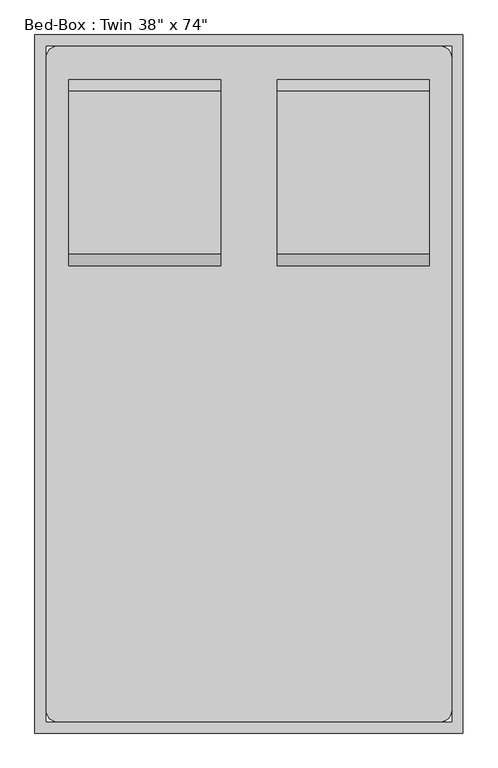
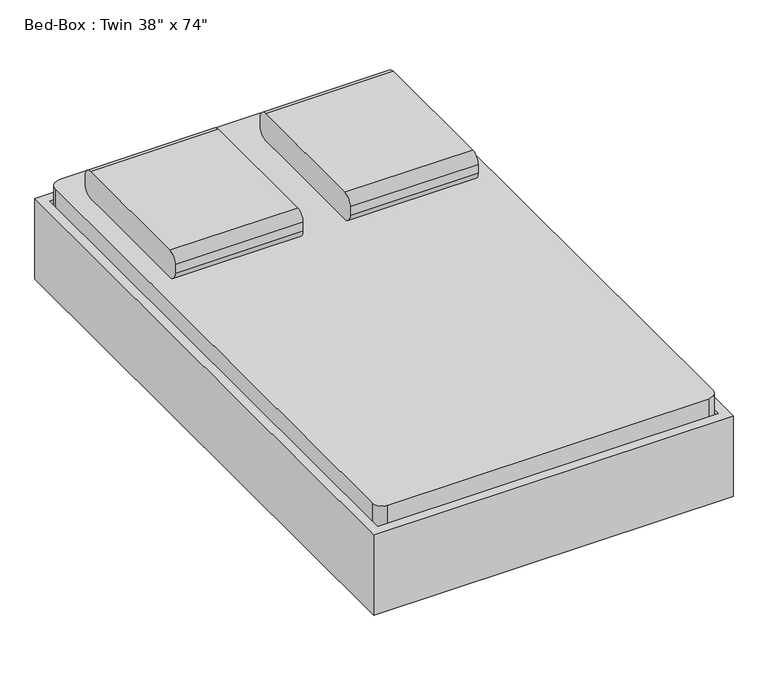
"""IFC4 building model written with IfcOpenShell, lengths in millimetres: furniture geometry."""

from ifc_helpers import new_model, si_unit, point, frame, frame_2d, origin, place, context, project, spatial, polyline, circle_curve, trimmed, segment, composite_curve, outline, extrude, source, transform, mapped, element, save
from ifc_brep_helpers import plane_surface, cylinder_surface, revolved_surface, advanced_brep


def furniture_631c00ae(model_context):
    return source(origin(), model_context, "Body", "SolidModel", [
        extrude(outline(composite_curve([segment(polyline([(425.9704918, 406.4), (57.6704918, 406.4)]), True, "CONTINUOUS"), segment(trimmed(circle_curve(frame_2d((57.6704918, 431.8)), 25.4), [point((57.6704918, 406.4))], [point((32.2704918, 431.8))], False, "CARTESIAN"), True, "CONTINUOUS"), segment(polyline([(32.2704918, 431.8), (32.2704918, 457.2)]), True, "CONTINUOUS"), segment(trimmed(circle_curve(frame_2d((57.6704918, 457.2)), 25.4), [point((32.2704918, 457.2))], [point((57.6704918, 482.6))], False, "CARTESIAN"), True, "CONTINUOUS"), segment(polyline([(57.6704918, 482.6), (425.9704918, 482.6)]), True, "CONTINUOUS"), segment(trimmed(circle_curve(frame_2d((425.9704918, 457.2)), 25.4), [point((425.9704918, 482.6))], [point((451.3704918, 457.2))], False, "CARTESIAN"), True, "CONTINUOUS"), segment(polyline([(451.3704918, 457.2), (451.3704918, 431.8)]), True, "CONTINUOUS"), segment(trimmed(circle_curve(frame_2d((425.9704918, 431.8)), 25.4), [point((451.3704918, 431.8))], [point((425.9704918, 406.4))], False, "CARTESIAN"), True, "CONTINUOUS")], self_intersect=False)), frame((402.652459, 0.0, 0.0), z_axis=(1.0, 0.0, 0.0), x_axis=(0.0, 1.0, 0.0)), (0.0, 0.0, 1.0), 342.9),
        extrude(outline(composite_curve([segment(polyline([(425.9704918, 406.4), (57.6704918, 406.4)]), True, "CONTINUOUS"), segment(trimmed(circle_curve(frame_2d((57.6704918, 431.8)), 25.4), [point((57.6704918, 406.4))], [point((32.2704918, 431.8))], False, "CARTESIAN"), True, "CONTINUOUS"), segment(polyline([(32.2704918, 431.8), (32.2704918, 457.2)]), True, "CONTINUOUS"), segment(trimmed(circle_curve(frame_2d((57.6704918, 457.2)), 25.4), [point((32.2704918, 457.2))], [point((57.6704918, 482.6))], False, "CARTESIAN"), True, "CONTINUOUS"), segment(polyline([(57.6704918, 482.6), (425.9704918, 482.6)]), True, "CONTINUOUS"), segment(trimmed(circle_curve(frame_2d((425.9704918, 457.2)), 25.4), [point((425.9704918, 482.6))], [point((451.3704918, 457.2))], False, "CARTESIAN"), True, "CONTINUOUS"), segment(polyline([(451.3704918, 457.2), (451.3704918, 431.8)]), True, "CONTINUOUS"), segment(trimmed(circle_curve(frame_2d((425.9704918, 431.8)), 25.4), [point((451.3704918, 431.8))], [point((425.9704918, 406.4))], False, "CARTESIAN"), True, "CONTINUOUS")], self_intersect=False)), frame((-67.247541, 0.0, 0.0), z_axis=(1.0, 0.0, 0.0), x_axis=(0.0, 1.0, 0.0)), (0.0, 0.0, 1.0), 342.9),
        advanced_brep(
        [(-117.7231784, 298.9704918, 177.8), (-117.7231784, 222.7704918, 177.8), (-117.7231784, 222.7704918, 196.85), (-117.7231784, 298.9704918, 196.85), (-66.9231784, 298.9704918, 177.8), (-66.9231784, 222.7704918, 177.8), (-54.7869899, 222.7704918, 196.85), (-54.7869899, 298.9704918, 196.85), (9.1476901, 298.9704918, 14.6654962), (9.1476901, 222.7704918, 14.6654962), (26.4128534, 222.7704918, 22.716374), (26.4128534, 298.9704918, 22.716374), (32.1679079, 222.7704918, 0.0), (32.1679079, 298.9704918, 0.0), (32.1679079, 222.7704918, 19.05), (32.1679079, 298.9704918, 19.05), (110.7804138, 298.9704918, 0.0), (110.7804138, 222.7704918, 0.0), (110.7804138, 222.7704918, 19.05), (110.7804138, 298.9704918, 19.05), (123.4804138, 222.7704918, 3.4029547), (123.4804138, 298.9704918, 3.4029547), (113.9554138, 222.7704918, 19.9007387), (113.9554138, 298.9704918, 19.9007387), (183.577459, 298.9704918, 38.1), (183.577459, 222.7704918, 38.1), (178.4730269, 222.7704918, 57.15), (178.4730269, 298.9704918, 57.15), (495.0518216, 298.9704918, 38.1), (495.0518216, 222.7704918, 38.1), (500.1562537, 222.7704918, 57.15), (500.1562537, 298.9704918, 57.15), (555.1488669, 298.9704918, 3.4029547), (555.1488669, 222.7704918, 3.4029547), (564.6738669, 222.7704918, 19.9007387), (564.6738669, 298.9704918, 19.9007387), (567.8488669, 222.7704918, 0.0), (567.8488669, 298.9704918, 0.0), (567.8488669, 222.7704918, 19.05), (567.8488669, 298.9704918, 19.05), (646.4613728, 298.9704918, 0.0), (646.4613728, 222.7704918, 0.0), (646.4613728, 222.7704918, 19.05), (646.4613728, 298.9704918, 19.05), (669.4815906, 222.7704918, 14.6654962), (669.4815906, 298.9704918, 14.6654962), (652.2164272, 222.7704918, 22.716374), (652.2164272, 298.9704918, 22.716374), (745.552459, 298.9704918, 177.8), (745.552459, 222.7704918, 177.8), (733.4162705, 222.7704918, 196.85), (733.4162705, 298.9704918, 196.85), (796.352459, 298.9704918, 177.8), (796.352459, 298.9704918, 196.85), (796.352459, 222.7704918, 196.85), (796.352459, 222.7704918, 177.8)],
        [
            (0, 1),
            (1, 2),
            (2, 3),
            (3, 0),
            (0, 4),
            (4, 5),
            (5, 1),
            (5, 6),
            (6, 2),
            (6, 7),
            (7, 3),
            (7, 4),
            (4, 8),
            (8, 9),
            (9, 5),
            (9, 10),
            (10, 6),
            (10, 11),
            (11, 7),
            (11, 8),
            (12, 9, circle_curve(frame((32.1679079, 222.7704918, 25.4), z_axis=(0.0, 1.0, 0.0), x_axis=(-0.9063077870366486, 0.0, -0.42261826174070233)), 25.4)),
            (8, 13, circle_curve(frame((32.1679079, 298.9704918, 25.4), z_axis=(0.0, -1.0, 0.0), x_axis=(-0.9063077870366486, 0.0, -0.42261826174070233)), 25.4)),
            (13, 12),
            (14, 10, circle_curve(frame((32.1679079, 222.7704918, 25.4), z_axis=(0.0, 1.0, 0.0), x_axis=(-0.9063077870366486, 0.0, -0.42261826174070233)), 6.35)),
            (12, 14),
            (15, 11, circle_curve(frame((32.1679079, 298.9704918, 25.4), z_axis=(0.0, 1.0, 0.0), x_axis=(-0.9063077870366486, 0.0, -0.42261826174070233)), 6.35)),
            (14, 15),
            (15, 13),
            (13, 16),
            (16, 17),
            (17, 12),
            (17, 18),
            (18, 14),
            (18, 19),
            (19, 15),
            (19, 16),
            (20, 17, circle_curve(frame((110.7804138, 222.7704918, 25.4), z_axis=(0.0, 1.0, 0.0), x_axis=(0.0, 0.0, -1.0)), 25.4)),
            (16, 21, circle_curve(frame((110.7804138, 298.9704918, 25.4), z_axis=(0.0, -1.0, 0.0), x_axis=(0.0, 0.0, -1.0)), 25.4)),
            (21, 20),
            (22, 18, circle_curve(frame((110.7804138, 222.7704918, 25.4), z_axis=(0.0, 1.0, 0.0), x_axis=(0.0, 0.0, -1.0)), 6.35)),
            (20, 22),
            (23, 19, circle_curve(frame((110.7804138, 298.9704918, 25.4), z_axis=(0.0, 1.0, 0.0), x_axis=(0.0, 0.0, -1.0)), 6.35)),
            (22, 23),
            (23, 21),
            (21, 24),
            (24, 25),
            (25, 20),
            (25, 26),
            (26, 22),
            (26, 27),
            (27, 23),
            (27, 24),
            (24, 28),
            (28, 29),
            (29, 25),
            (29, 30),
            (30, 26),
            (30, 31),
            (31, 27),
            (31, 28),
            (28, 32),
            (32, 33),
            (33, 29),
            (33, 34),
            (34, 30),
            (34, 35),
            (35, 31),
            (35, 32),
            (36, 33, circle_curve(frame((567.8488669, 222.7704918, 25.4), z_axis=(0.0, 1.0, 0.0), x_axis=(-0.5000000000000463, 0.0, -0.8660254037844118)), 25.4)),
            (32, 37, circle_curve(frame((567.8488669, 298.9704918, 25.4), z_axis=(0.0, -1.0, 0.0), x_axis=(-0.5000000000000463, 0.0, -0.8660254037844118)), 25.4)),
            (37, 36),
            (38, 34, circle_curve(frame((567.8488669, 222.7704918, 25.4), z_axis=(0.0, 1.0, 0.0), x_axis=(-0.5000000000000463, 0.0, -0.8660254037844118)), 6.35)),
            (36, 38),
            (39, 35, circle_curve(frame((567.8488669, 298.9704918, 25.4), z_axis=(0.0, 1.0, 0.0), x_axis=(-0.5000000000000463, 0.0, -0.8660254037844118)), 6.35)),
            (38, 39),
            (39, 37),
            (37, 40),
            (40, 41),
            (41, 36),
            (41, 42),
            (42, 38),
            (42, 43),
            (43, 39),
            (43, 40),
            (44, 41, circle_curve(frame((646.4613728, 222.7704918, 25.4), z_axis=(0.0, 1.0, 0.0), x_axis=(0.0, 0.0, -1.0)), 25.4)),
            (40, 45, circle_curve(frame((646.4613728, 298.9704918, 25.4), z_axis=(0.0, -1.0, 0.0), x_axis=(0.0, 0.0, -1.0)), 25.4)),
            (45, 44),
            (46, 42, circle_curve(frame((646.4613728, 222.7704918, 25.4), z_axis=(0.0, 1.0, 0.0), x_axis=(0.0, 0.0, -1.0)), 6.35)),
            (44, 46),
            (47, 43, circle_curve(frame((646.4613728, 298.9704918, 25.4), z_axis=(0.0, 1.0, 0.0), x_axis=(0.0, 0.0, -1.0)), 6.35)),
            (46, 47),
            (47, 45),
            (45, 48),
            (48, 49),
            (49, 44),
            (49, 50),
            (50, 46),
            (50, 51),
            (51, 47),
            (51, 48),
            (52, 53),
            (53, 54),
            (54, 55),
            (55, 52),
            (48, 52),
            (55, 49),
            (54, 50),
            (53, 51),
        ],
        [
            plane_surface(frame((-117.7231784, 552.9704918, -152.9490627), z_axis=(-1.0, 0.0, 0.0), x_axis=(0.0, 1.0, 0.0))),
            plane_surface(frame((-117.7231784, 298.9704918, 177.8), z_axis=(0.0, 0.0, -1.0), x_axis=(1.0, 0.0, 0.0))),
            plane_surface(frame((-117.7231784, 222.7704918, 177.8), z_axis=(0.0, -1.0, 0.0), x_axis=(1.0, 0.0, 0.0))),
            plane_surface(frame((-117.7231784, 222.7704918, 196.85), z_axis=(0.0, 0.0, 1.0), x_axis=(1.0, 0.0, 0.0))),
            plane_surface(frame((-117.7231784, 298.9704918, 196.85), z_axis=(0.0, 1.0, 0.0), x_axis=(1.0, 0.0, 0.0))),
            plane_surface(frame((-66.9231784, 298.9704918, 177.8), z_axis=(-0.9063077870366486, 0.0, -0.42261826174070244), x_axis=(0.42261826174070244, 0.0, -0.9063077870366486))),
            plane_surface(frame((-66.9231784, 222.7704918, 177.8), z_axis=(0.0, -1.0000000000000002, 0.0), x_axis=(0.4226182617407026, 0.0, -0.9063077870366486))),
            plane_surface(frame((-54.7869899, 222.7704918, 196.85), z_axis=(0.9063077870366485, 0.0, 0.4226182617407026), x_axis=(0.4226182617407026, 0.0, -0.9063077870366485))),
            plane_surface(frame((-54.7869899, 298.9704918, 196.85), z_axis=(0.0, 1.0000000000000002, 0.0), x_axis=(0.4226182617407026, 0.0, -0.9063077870366486))),
            cylinder_surface(frame((32.1679079, 552.9704918, 25.4), z_axis=(0.0, -1.0, 0.0), x_axis=(-0.9063077870366486, 0.0, -0.42261826174070233)), 25.4),
            plane_surface(frame((32.1679079, 222.7704918, 25.4), z_axis=(0.0, -1.0, 0.0), x_axis=(-0.9063077870366486, 0.0, -0.42261826174070233))),
            revolved_surface(polyline([(26.412853452317286, 222.7704918, 22.71637403794654), (26.412853452317286, 298.9704918, 22.71637403794654)]), (32.1679079, 552.9704918, 25.4), (0.0, -1.0, 0.0)),
            plane_surface(frame((32.1679079, 298.9704918, 25.4), z_axis=(0.0, 1.0, 0.0), x_axis=(-0.9063077870366486, 0.0, -0.42261826174070233))),
            plane_surface(frame((32.1679079, 298.9704918, 0.0), z_axis=(0.0, 0.0, -1.0), x_axis=(1.0, 0.0, 0.0))),
            plane_surface(frame((32.1679079, 222.7704918, 0.0), z_axis=(0.0, -1.0, 0.0), x_axis=(1.0, 0.0, 0.0))),
            plane_surface(frame((32.1679079, 222.7704918, 19.05), z_axis=(0.0, 0.0, 1.0), x_axis=(1.0, 0.0, 0.0))),
            plane_surface(frame((32.1679079, 298.9704918, 19.05), z_axis=(0.0, 1.0, 0.0), x_axis=(1.0, 0.0, 0.0))),
            cylinder_surface(frame((110.7804138, 552.9704918, 25.4), z_axis=(0.0, -1.0, 0.0), x_axis=(0.0, 0.0, -1.0)), 25.4),
            plane_surface(frame((110.7804138, 222.7704918, 25.4), z_axis=(0.0, -1.0, 0.0), x_axis=(0.0, 0.0, -1.0))),
            revolved_surface(polyline([(110.7804138, 222.7704918, 19.049999999999997), (110.7804138, 298.9704918, 19.049999999999997)]), (110.7804138, 552.9704918, 25.4), (0.0, -1.0, 0.0)),
            plane_surface(frame((110.7804138, 298.9704918, 25.4), z_axis=(0.0, 1.0, 0.0), x_axis=(0.0, 0.0, -1.0))),
            plane_surface(frame((123.4804138, 298.9704918, 3.4029547), z_axis=(0.49999999999987804, 0.0, -0.8660254037845091), x_axis=(0.8660254037845091, 0.0, 0.49999999999987804))),
            plane_surface(frame((123.4804138, 222.7704918, 3.4029547), z_axis=(0.0, -1.0, 0.0), x_axis=(0.8660254037845093, 0.0, 0.49999999999987765))),
            plane_surface(frame((113.9554138, 222.7704918, 19.9007387), z_axis=(-0.49999999999987815, 0.0, 0.8660254037845091), x_axis=(0.8660254037845091, 0.0, 0.49999999999987815))),
            plane_surface(frame((113.9554138, 298.9704918, 19.9007387), z_axis=(0.0, 1.0, 0.0), x_axis=(0.8660254037845092, 0.0, 0.49999999999987776))),
            plane_surface(frame((183.577459, 298.9704918, 38.1), z_axis=(0.0, 0.0, -1.0), x_axis=(1.0, 0.0, 0.0))),
            plane_surface(frame((183.577459, 222.7704918, 38.1), z_axis=(0.0, -1.0, 0.0), x_axis=(1.0, 0.0, 0.0))),
            plane_surface(frame((178.4730269, 222.7704918, 57.15), z_axis=(0.0, 0.0, 1.0), x_axis=(1.0, 0.0, 0.0))),
            plane_surface(frame((178.4730269, 298.9704918, 57.15), z_axis=(0.0, 1.0, 0.0), x_axis=(1.0, 0.0, 0.0))),
            plane_surface(frame((495.0518216, 298.9704918, 38.1), z_axis=(-0.5000000000000461, 0.0, -0.8660254037844122), x_axis=(0.8660254037844122, 0.0, -0.5000000000000461))),
            plane_surface(frame((495.0518216, 222.7704918, 38.1), z_axis=(0.0, -1.0, 0.0), x_axis=(0.8660254037844125, 0.0, -0.5000000000000454))),
            plane_surface(frame((500.1562537, 222.7704918, 57.15), z_axis=(0.5000000000000456, 0.0, 0.8660254037844124), x_axis=(0.8660254037844124, 0.0, -0.5000000000000456))),
            plane_surface(frame((500.1562537, 298.9704918, 57.15), z_axis=(0.0, 1.0, 0.0), x_axis=(0.8660254037844127, 0.0, -0.5000000000000449))),
            cylinder_surface(frame((567.8488669, 552.9704918, 25.4), z_axis=(0.0, -1.0, 0.0), x_axis=(-0.5000000000000463, 0.0, -0.8660254037844118)), 25.4),
            plane_surface(frame((567.8488669, 222.7704918, 25.4), z_axis=(0.0, -1.0000000000000002, 0.0), x_axis=(-0.5000000000000464, 0.0, -0.866025403784412))),
            revolved_surface(polyline([(564.6738668999997, 222.7704918, 19.90073868596898), (564.6738668999997, 298.9704918, 19.90073868596898)]), (567.8488669, 552.9704918, 25.4), (0.0, -1.0, 0.0)),
            plane_surface(frame((567.8488669, 298.9704918, 25.4), z_axis=(0.0, 1.0000000000000002, 0.0), x_axis=(-0.5000000000000464, 0.0, -0.866025403784412))),
            plane_surface(frame((567.8488669, 298.9704918, 0.0), z_axis=(0.0, 0.0, -1.0), x_axis=(1.0, 0.0, 0.0))),
            plane_surface(frame((567.8488669, 222.7704918, 0.0), z_axis=(0.0, -1.0, 0.0), x_axis=(1.0, 0.0, 0.0))),
            plane_surface(frame((567.8488669, 222.7704918, 19.05), z_axis=(0.0, 0.0, 1.0), x_axis=(1.0, 0.0, 0.0))),
            plane_surface(frame((567.8488669, 298.9704918, 19.05), z_axis=(0.0, 1.0, 0.0), x_axis=(1.0, 0.0, 0.0))),
            cylinder_surface(frame((646.4613728, 552.9704918, 25.4), z_axis=(0.0, -1.0, 0.0), x_axis=(0.0, 0.0, -1.0)), 25.4),
            plane_surface(frame((646.4613728, 222.7704918, 25.4), z_axis=(0.0, -1.0, 0.0), x_axis=(0.0, 0.0, -1.0))),
            revolved_surface(polyline([(646.4613728, 222.7704918, 19.049999999999997), (646.4613728, 298.9704918, 19.049999999999997)]), (646.4613728, 552.9704918, 25.4), (0.0, -1.0, 0.0)),
            plane_surface(frame((646.4613728, 298.9704918, 25.4), z_axis=(0.0, 1.0, 0.0), x_axis=(0.0, 0.0, -1.0))),
            plane_surface(frame((669.4815906, 298.9704918, 14.6654962), z_axis=(0.90630778703668, 0.0, -0.42261826174063516), x_axis=(0.42261826174063516, 0.0, 0.90630778703668))),
            plane_surface(frame((669.4815906, 222.7704918, 14.6654962), z_axis=(0.0, -1.0, 0.0), x_axis=(0.422618261740635, 0.0, 0.90630778703668))),
            plane_surface(frame((652.2164272, 222.7704918, 22.716374), z_axis=(-0.9063077870366799, 0.0, 0.42261826174063544), x_axis=(0.42261826174063544, 0.0, 0.9063077870366799))),
            plane_surface(frame((652.2164272, 298.9704918, 22.716374), z_axis=(0.0, 1.0, 0.0), x_axis=(0.4226182617406361, 0.0, 0.9063077870366795))),
            plane_surface(frame((796.352459, 552.9704918, -152.9490627), z_axis=(1.0, 0.0, 0.0), x_axis=(0.0, 1.0, 0.0))),
            plane_surface(frame((745.552459, 298.9704918, 177.8), z_axis=(0.0, 0.0, -1.0), x_axis=(1.0, 0.0, 0.0))),
            plane_surface(frame((745.552459, 222.7704918, 177.8), z_axis=(0.0, -1.0, 0.0), x_axis=(1.0, 0.0, 0.0))),
            plane_surface(frame((733.4162705, 222.7704918, 196.85), z_axis=(0.0, 0.0, 1.0), x_axis=(1.0, 0.0, 0.0))),
            plane_surface(frame((733.4162705, 298.9704918, 196.85), z_axis=(0.0, 1.0, 0.0), x_axis=(1.0, 0.0, 0.0))),
        ],
        [
            (0, [[1, 2, 3, 4]]),
            (1, [[-1, 5, 6, 7]]),
            (2, [[-2, -7, 8, 9]]),
            (3, [[-3, -9, 10, 11]]),
            (4, [[-4, -11, 12, -5]]),
            (5, [[-6, 13, 14, 15]]),
            (6, [[-8, -15, 16, 17]]),
            (7, [[-10, -17, 18, 19]]),
            (8, [[-12, -19, 20, -13]]),
            (9, [[21, -14, 22, 23]]),
            (10, [[24, -16, -21, 25]]),
            (11, [[26, -18, -24, 27]]),
            (12, [[-22, -20, -26, 28]]),
            (13, [[-23, 29, 30, 31]]),
            (14, [[-25, -31, 32, 33]]),
            (15, [[-27, -33, 34, 35]]),
            (16, [[-28, -35, 36, -29]]),
            (17, [[37, -30, 38, 39]]),
            (18, [[40, -32, -37, 41]]),
            (19, [[42, -34, -40, 43]]),
            (20, [[-38, -36, -42, 44]]),
            (21, [[-39, 45, 46, 47]]),
            (22, [[-41, -47, 48, 49]]),
            (23, [[-43, -49, 50, 51]]),
            (24, [[-44, -51, 52, -45]]),
            (25, [[-46, 53, 54, 55]]),
            (26, [[-48, -55, 56, 57]]),
            (27, [[-50, -57, 58, 59]]),
            (28, [[-52, -59, 60, -53]]),
            (29, [[-54, 61, 62, 63]]),
            (30, [[-56, -63, 64, 65]]),
            (31, [[-58, -65, 66, 67]]),
            (32, [[-60, -67, 68, -61]]),
            (33, [[69, -62, 70, 71]]),
            (34, [[72, -64, -69, 73]]),
            (35, [[74, -66, -72, 75]]),
            (36, [[-70, -68, -74, 76]]),
            (37, [[-71, 77, 78, 79]]),
            (38, [[-73, -79, 80, 81]]),
            (39, [[-75, -81, 82, 83]]),
            (40, [[-76, -83, 84, -77]]),
            (41, [[85, -78, 86, 87]]),
            (42, [[88, -80, -85, 89]]),
            (43, [[90, -82, -88, 91]]),
            (44, [[-86, -84, -90, 92]]),
            (45, [[-87, 93, 94, 95]]),
            (46, [[-89, -95, 96, 97]]),
            (47, [[-91, -97, 98, 99]]),
            (48, [[-92, -99, 100, -93]]),
            (49, [[101, 102, 103, 104]]),
            (50, [[-94, 105, -104, 106]]),
            (51, [[-96, -106, -103, 107]]),
            (52, [[-98, -107, -102, 108]]),
            (53, [[-100, -108, -101, -105]]),
        ],
    ),
        extrude(outline(composite_curve([segment(polyline([(-92.647541, 527.5704918), (770.952459, 527.5704918)]), True, "CONTINUOUS"), segment(trimmed(circle_curve(frame_2d((770.952459, 502.1704918)), 25.4), [point((770.952459, 527.5704918))], [point((796.352459, 502.1704918))], False, "CARTESIAN"), True, "CONTINUOUS"), segment(polyline([(796.352459, 502.1704918), (796.352459, -971.0295082)]), True, "CONTINUOUS"), segment(trimmed(circle_curve(frame_2d((770.952459, -971.0295082)), 25.4), [point((796.352459, -971.0295082))], [point((770.952459, -996.4295082))], False, "CARTESIAN"), True, "CONTINUOUS"), segment(polyline([(770.952459, -996.4295082), (-92.647541, -996.4295082)]), True, "CONTINUOUS"), segment(trimmed(circle_curve(frame_2d((-92.647541, -971.0295082)), 25.4), [point((-92.647541, -996.4295082))], [point((-118.047541, -971.0295082))], False, "CARTESIAN"), True, "CONTINUOUS"), segment(polyline([(-118.047541, -971.0295082), (-118.047541, 502.1704918)]), True, "CONTINUOUS"), segment(trimmed(circle_curve(frame_2d((-92.647541, 502.1704918)), 25.4), [point((-118.047541, 502.1704918))], [point((-92.647541, 527.5704918))], False, "CARTESIAN"), True, "CONTINUOUS")], self_intersect=False)), frame((0.0, 0.0, 203.2), z_axis=(0.0, 0.0, 1.0), x_axis=(1.0, 0.0, 0.0)), (0.0, 0.0, 1.0), 203.2),
        advanced_brep(
        [(-118.047541, -717.0295082, 196.85), (-118.047541, -717.0295082, 177.8), (-118.047541, -793.2295082, 177.8), (-118.047541, -793.2295082, 196.85), (-55.1113525, -717.0295082, 196.85), (-67.247541, -717.0295082, 177.8), (-67.247541, -793.2295082, 177.8), (-55.1113525, -793.2295082, 196.85), (26.0884908, -717.0295082, 22.716374), (8.8233275, -717.0295082, 14.6654962), (8.8233275, -793.2295082, 14.6654962), (26.0884908, -793.2295082, 22.716374), (31.8435453, -717.0295082, 0.0), (31.8435453, -717.0295082, 19.05), (31.8435453, -793.2295082, 0.0), (31.8435453, -793.2295082, 19.05), (110.4560511, -717.0295082, 19.05), (110.4560511, -717.0295082, 0.0), (110.4560511, -793.2295082, 0.0), (110.4560511, -793.2295082, 19.05), (123.1560511, -717.0295082, 3.4029547), (113.6310511, -717.0295082, 19.9007387), (123.1560511, -793.2295082, 3.4029547), (113.6310511, -793.2295082, 19.9007387), (178.1486643, -717.0295082, 57.15), (183.2530964, -717.0295082, 38.1), (183.2530964, -793.2295082, 38.1), (178.1486643, -793.2295082, 57.15), (500.1562537, -717.0295082, 57.15), (495.0518216, -717.0295082, 38.1), (495.0518216, -793.2295082, 38.1), (500.1562537, -793.2295082, 57.15), (564.6738669, -717.0295082, 19.9007387), (555.1488669, -717.0295082, 3.4029547), (555.1488669, -793.2295082, 3.4029547), (564.6738669, -793.2295082, 19.9007387), (567.8488669, -717.0295082, 0.0), (567.8488669, -717.0295082, 19.05), (567.8488669, -793.2295082, 0.0), (567.8488669, -793.2295082, 19.05), (646.4613728, -717.0295082, 19.05), (646.4613728, -717.0295082, 0.0), (646.4613728, -793.2295082, 0.0), (646.4613728, -793.2295082, 19.05), (669.4815906, -717.0295082, 14.6654962), (652.2164272, -717.0295082, 22.716374), (669.4815906, -793.2295082, 14.6654962), (652.2164272, -793.2295082, 22.716374), (733.4162705, -717.0295082, 196.85), (745.552459, -717.0295082, 177.8), (745.552459, -793.2295082, 177.8), (733.4162705, -793.2295082, 196.85), (796.352459, -717.0295082, 196.85), (796.352459, -793.2295082, 196.85), (796.352459, -793.2295082, 177.8), (796.352459, -717.0295082, 177.8)],
        [
            (0, 1),
            (1, 2),
            (2, 3),
            (3, 0),
            (0, 4),
            (4, 5),
            (5, 1),
            (5, 6),
            (6, 2),
            (6, 7),
            (7, 3),
            (7, 4),
            (4, 8),
            (8, 9),
            (9, 5),
            (9, 10),
            (10, 6),
            (10, 11),
            (11, 7),
            (11, 8),
            (12, 9, circle_curve(frame((31.8435453, -717.0295082, 25.4), z_axis=(0.0, 1.0, 0.0), x_axis=(-0.906307787036663, 0.0, -0.4226182617406713)), 25.4)),
            (8, 13, circle_curve(frame((31.8435453, -717.0295082, 25.4), z_axis=(0.0, -1.0, 0.0), x_axis=(-0.906307787036663, 0.0, -0.4226182617406713)), 6.35)),
            (13, 12),
            (14, 10, circle_curve(frame((31.8435453, -793.2295082, 25.4), z_axis=(0.0, 1.0, 0.0), x_axis=(-0.906307787036663, 0.0, -0.4226182617406713)), 25.4)),
            (12, 14),
            (15, 11, circle_curve(frame((31.8435453, -793.2295082, 25.4), z_axis=(0.0, 1.0, 0.0), x_axis=(-0.906307787036663, 0.0, -0.4226182617406713)), 6.35)),
            (14, 15),
            (15, 13),
            (13, 16),
            (16, 17),
            (17, 12),
            (17, 18),
            (18, 14),
            (18, 19),
            (19, 15),
            (19, 16),
            (20, 17, circle_curve(frame((110.4560511, -717.0295082, 25.4), z_axis=(0.0, 1.0, 0.0), x_axis=(0.0, 0.0, -1.0)), 25.4)),
            (16, 21, circle_curve(frame((110.4560511, -717.0295082, 25.4), z_axis=(0.0, -1.0, 0.0), x_axis=(0.0, 0.0, -1.0)), 6.35)),
            (21, 20),
            (22, 18, circle_curve(frame((110.4560511, -793.2295082, 25.4), z_axis=(0.0, 1.0, 0.0), x_axis=(0.0, 0.0, -1.0)), 25.4)),
            (20, 22),
            (23, 19, circle_curve(frame((110.4560511, -793.2295082, 25.4), z_axis=(0.0, 1.0, 0.0), x_axis=(0.0, 0.0, -1.0)), 6.35)),
            (22, 23),
            (23, 21),
            (21, 24),
            (24, 25),
            (25, 20),
            (25, 26),
            (26, 22),
            (26, 27),
            (27, 23),
            (27, 24),
            (24, 28),
            (28, 29),
            (29, 25),
            (29, 30),
            (30, 26),
            (30, 31),
            (31, 27),
            (31, 28),
            (28, 32),
            (32, 33),
            (33, 29),
            (33, 34),
            (34, 30),
            (34, 35),
            (35, 31),
            (35, 32),
            (36, 33, circle_curve(frame((567.8488669, -717.0295082, 25.4), z_axis=(0.0, 1.0, 0.0), x_axis=(-0.5000000000000479, 0.0, -0.866025403784411)), 25.4)),
            (32, 37, circle_curve(frame((567.8488669, -717.0295082, 25.4), z_axis=(0.0, -1.0, 0.0), x_axis=(-0.5000000000000479, 0.0, -0.866025403784411)), 6.35)),
            (37, 36),
            (38, 34, circle_curve(frame((567.8488669, -793.2295082, 25.4), z_axis=(0.0, 1.0, 0.0), x_axis=(-0.5000000000000479, 0.0, -0.866025403784411)), 25.4)),
            (36, 38),
            (39, 35, circle_curve(frame((567.8488669, -793.2295082, 25.4), z_axis=(0.0, 1.0, 0.0), x_axis=(-0.5000000000000479, 0.0, -0.866025403784411)), 6.35)),
            (38, 39),
            (39, 37),
            (37, 40),
            (40, 41),
            (41, 36),
            (41, 42),
            (42, 38),
            (42, 43),
            (43, 39),
            (43, 40),
            (44, 41, circle_curve(frame((646.4613728, -717.0295082, 25.4), z_axis=(0.0, 1.0, 0.0), x_axis=(0.0, 0.0, -1.0)), 25.4)),
            (40, 45, circle_curve(frame((646.4613728, -717.0295082, 25.4), z_axis=(0.0, -1.0, 0.0), x_axis=(0.0, 0.0, -1.0)), 6.35)),
            (45, 44),
            (46, 42, circle_curve(frame((646.4613728, -793.2295082, 25.4), z_axis=(0.0, 1.0, 0.0), x_axis=(0.0, 0.0, -1.0)), 25.4)),
            (44, 46),
            (47, 43, circle_curve(frame((646.4613728, -793.2295082, 25.4), z_axis=(0.0, 1.0, 0.0), x_axis=(0.0, 0.0, -1.0)), 6.35)),
            (46, 47),
            (47, 45),
            (45, 48),
            (48, 49),
            (49, 44),
            (49, 50),
            (50, 46),
            (50, 51),
            (51, 47),
            (51, 48),
            (52, 53),
            (53, 54),
            (54, 55),
            (55, 52),
            (48, 52),
            (55, 49),
            (54, 50),
            (53, 51),
        ],
        [
            plane_surface(frame((-118.047541, -1021.8295082, -127.5947323), z_axis=(-1.0, 0.0, 0.0), x_axis=(0.0, 1.0, 0.0))),
            plane_surface(frame((-118.047541, -717.0295082, 196.85), z_axis=(0.0, 1.0, 0.0), x_axis=(1.0, 0.0, 0.0))),
            plane_surface(frame((-118.047541, -717.0295082, 177.8), z_axis=(0.0, 0.0, -1.0), x_axis=(1.0, 0.0, 0.0))),
            plane_surface(frame((-118.047541, -793.2295082, 177.8), z_axis=(0.0, -1.0, 0.0), x_axis=(1.0, 0.0, 0.0))),
            plane_surface(frame((-118.047541, -793.2295082, 196.85), z_axis=(0.0, 0.0, 1.0), x_axis=(1.0, 0.0, 0.0))),
            plane_surface(frame((-55.1113525, -717.0295082, 196.85), z_axis=(0.0, 1.0000000000000002, 0.0), x_axis=(0.42261826174067113, 0.0, -0.9063077870366633))),
            plane_surface(frame((-67.247541, -717.0295082, 177.8), z_axis=(-0.9063077870366633, 0.0, -0.42261826174067096), x_axis=(0.42261826174067096, 0.0, -0.9063077870366633))),
            plane_surface(frame((-67.247541, -793.2295082, 177.8), z_axis=(0.0, -1.0, 0.0), x_axis=(0.4226182617406711, 0.0, -0.9063077870366631))),
            plane_surface(frame((-55.1113525, -793.2295082, 196.85), z_axis=(0.906307787036663, 0.0, 0.4226182617406714), x_axis=(0.4226182617406714, 0.0, -0.906307787036663))),
            plane_surface(frame((31.8435453, -717.0295082, 25.4), z_axis=(0.0, 1.0, 0.0), x_axis=(-0.906307787036663, 0.0, -0.4226182617406713))),
            cylinder_surface(frame((31.8435453, -1021.8295082, 25.4), z_axis=(0.0, -1.0, 0.0), x_axis=(-0.906307787036663, 0.0, -0.4226182617406713)), 25.4),
            plane_surface(frame((31.8435453, -793.2295082, 25.4), z_axis=(0.0, -1.0, 0.0), x_axis=(-0.906307787036663, 0.0, -0.4226182617406713))),
            revolved_surface(polyline([(26.08849085231719, -793.2295082, 22.716374037946736), (26.08849085231719, -717.0295082, 22.716374037946736)]), (31.8435453, -1021.8295082, 25.4), (0.0, -1.0, 0.0)),
            plane_surface(frame((31.8435453, -717.0295082, 19.05), z_axis=(0.0, 1.0, 0.0), x_axis=(1.0, 0.0, 0.0))),
            plane_surface(frame((31.8435453, -717.0295082, 0.0), z_axis=(0.0, 0.0, -1.0), x_axis=(1.0, 0.0, 0.0))),
            plane_surface(frame((31.8435453, -793.2295082, 0.0), z_axis=(0.0, -1.0, 0.0), x_axis=(1.0, 0.0, 0.0))),
            plane_surface(frame((31.8435453, -793.2295082, 19.05), z_axis=(0.0, 0.0, 1.0), x_axis=(1.0, 0.0, 0.0))),
            plane_surface(frame((110.4560511, -717.0295082, 25.4), z_axis=(0.0, 1.0, 0.0), x_axis=(0.0, 0.0, -1.0))),
            cylinder_surface(frame((110.4560511, -1021.8295082, 25.4), z_axis=(0.0, -1.0, 0.0), x_axis=(0.0, 0.0, -1.0)), 25.4),
            plane_surface(frame((110.4560511, -793.2295082, 25.4), z_axis=(0.0, -1.0, 0.0), x_axis=(0.0, 0.0, -1.0))),
            revolved_surface(polyline([(110.4560511, -793.2295082, 19.049999999999997), (110.4560511, -717.0295082, 19.049999999999997)]), (110.4560511, -1021.8295082, 25.4), (0.0, -1.0, 0.0)),
            plane_surface(frame((113.6310511, -717.0295082, 19.9007387), z_axis=(0.0, 1.0, 0.0), x_axis=(0.8660254037844787, 0.0, 0.4999999999999308))),
            plane_surface(frame((123.1560511, -717.0295082, 3.4029547), z_axis=(0.4999999999999308, 0.0, -0.8660254037844786), x_axis=(0.8660254037844786, 0.0, 0.4999999999999308))),
            plane_surface(frame((123.1560511, -793.2295082, 3.4029547), z_axis=(0.0, -1.0, 0.0), x_axis=(0.8660254037844786, 0.0, 0.49999999999993083))),
            plane_surface(frame((113.6310511, -793.2295082, 19.9007387), z_axis=(-0.4999999999999306, 0.0, 0.8660254037844788), x_axis=(0.8660254037844788, 0.0, 0.4999999999999306))),
            plane_surface(frame((178.1486643, -717.0295082, 57.15), z_axis=(0.0, 1.0, 0.0), x_axis=(1.0, 0.0, 0.0))),
            plane_surface(frame((183.2530964, -717.0295082, 38.1), z_axis=(0.0, 0.0, -1.0), x_axis=(1.0, 0.0, 0.0))),
            plane_surface(frame((183.2530964, -793.2295082, 38.1), z_axis=(0.0, -1.0, 0.0), x_axis=(1.0, 0.0, 0.0))),
            plane_surface(frame((178.1486643, -793.2295082, 57.15), z_axis=(0.0, 0.0, 1.0), x_axis=(1.0, 0.0, 0.0))),
            plane_surface(frame((500.1562537, -717.0295082, 57.15), z_axis=(0.0, 1.0, 0.0), x_axis=(0.8660254037844095, 0.0, -0.5000000000000506))),
            plane_surface(frame((495.0518216, -717.0295082, 38.1), z_axis=(-0.5000000000000508, 0.0, -0.8660254037844094), x_axis=(0.8660254037844094, 0.0, -0.5000000000000508))),
            plane_surface(frame((495.0518216, -793.2295082, 38.1), z_axis=(0.0, -1.0, 0.0), x_axis=(0.8660254037844094, 0.0, -0.5000000000000506))),
            plane_surface(frame((500.1562537, -793.2295082, 57.15), z_axis=(0.5000000000000505, 0.0, 0.8660254037844095), x_axis=(0.8660254037844095, 0.0, -0.5000000000000505))),
            plane_surface(frame((567.8488669, -717.0295082, 25.4), z_axis=(0.0, 1.0000000000000002, 0.0), x_axis=(-0.500000000000048, 0.0, -0.8660254037844111))),
            cylinder_surface(frame((567.8488669, -1021.8295082, 25.4), z_axis=(0.0, -1.0, 0.0), x_axis=(-0.5000000000000479, 0.0, -0.866025403784411)), 25.4),
            plane_surface(frame((567.8488669, -793.2295082, 25.4), z_axis=(0.0, -1.0000000000000002, 0.0), x_axis=(-0.500000000000048, 0.0, -0.8660254037844111))),
            revolved_surface(polyline([(564.6738668999997, -793.2295082, 19.90073868596899), (564.6738668999997, -717.0295082, 19.90073868596899)]), (567.8488669, -1021.8295082, 25.4), (0.0, -1.0, 0.0)),
            plane_surface(frame((567.8488669, -717.0295082, 19.05), z_axis=(0.0, 1.0, 0.0), x_axis=(1.0, 0.0, 0.0))),
            plane_surface(frame((567.8488669, -717.0295082, 0.0), z_axis=(0.0, 0.0, -1.0), x_axis=(1.0, 0.0, 0.0))),
            plane_surface(frame((567.8488669, -793.2295082, 0.0), z_axis=(0.0, -1.0, 0.0), x_axis=(1.0, 0.0, 0.0))),
            plane_surface(frame((567.8488669, -793.2295082, 19.05), z_axis=(0.0, 0.0, 1.0), x_axis=(1.0, 0.0, 0.0))),
            plane_surface(frame((646.4613728, -717.0295082, 25.4), z_axis=(0.0, 1.0, 0.0), x_axis=(0.0, 0.0, -1.0))),
            cylinder_surface(frame((646.4613728, -1021.8295082, 25.4), z_axis=(0.0, -1.0, 0.0), x_axis=(0.0, 0.0, -1.0)), 25.4),
            plane_surface(frame((646.4613728, -793.2295082, 25.4), z_axis=(0.0, -1.0, 0.0), x_axis=(0.0, 0.0, -1.0))),
            revolved_surface(polyline([(646.4613728, -793.2295082, 19.049999999999997), (646.4613728, -717.0295082, 19.049999999999997)]), (646.4613728, -1021.8295082, 25.4), (0.0, -1.0, 0.0)),
            plane_surface(frame((652.2164272, -717.0295082, 22.716374), z_axis=(0.0, 1.0000000000000002, 0.0), x_axis=(0.42261826174054085, 0.0, 0.906307787036724))),
            plane_surface(frame((669.4815906, -717.0295082, 14.6654962), z_axis=(0.9063077870367241, 0.0, -0.4226182617405405), x_axis=(0.4226182617405405, 0.0, 0.9063077870367241))),
            plane_surface(frame((669.4815906, -793.2295082, 14.6654962), z_axis=(0.0, -1.0, 0.0), x_axis=(0.42261826174054046, 0.0, 0.9063077870367241))),
            plane_surface(frame((652.2164272, -793.2295082, 22.716374), z_axis=(-0.906307787036724, 0.0, 0.42261826174054085), x_axis=(0.42261826174054085, 0.0, 0.906307787036724))),
            plane_surface(frame((796.352459, -1021.8295082, -127.5947323), z_axis=(1.0, 0.0, 0.0), x_axis=(0.0, 1.0, 0.0))),
            plane_surface(frame((733.4162705, -717.0295082, 196.85), z_axis=(0.0, 1.0, 0.0), x_axis=(1.0, 0.0, 0.0))),
            plane_surface(frame((745.552459, -717.0295082, 177.8), z_axis=(0.0, 0.0, -1.0), x_axis=(1.0, 0.0, 0.0))),
            plane_surface(frame((745.552459, -793.2295082, 177.8), z_axis=(0.0, -1.0, 0.0), x_axis=(1.0, 0.0, 0.0))),
            plane_surface(frame((733.4162705, -793.2295082, 196.85), z_axis=(0.0, 0.0, 1.0), x_axis=(1.0, 0.0, 0.0))),
        ],
        [
            (0, [[1, 2, 3, 4]]),
            (1, [[-1, 5, 6, 7]]),
            (2, [[-2, -7, 8, 9]]),
            (3, [[-3, -9, 10, 11]]),
            (4, [[-4, -11, 12, -5]]),
            (5, [[-6, 13, 14, 15]]),
            (6, [[-8, -15, 16, 17]]),
            (7, [[-10, -17, 18, 19]]),
            (8, [[-12, -19, 20, -13]]),
            (9, [[21, -14, 22, 23]]),
            (10, [[24, -16, -21, 25]]),
            (11, [[26, -18, -24, 27]]),
            (12, [[-22, -20, -26, 28]]),
            (13, [[-23, 29, 30, 31]]),
            (14, [[-25, -31, 32, 33]]),
            (15, [[-27, -33, 34, 35]]),
            (16, [[-28, -35, 36, -29]]),
            (17, [[37, -30, 38, 39]]),
            (18, [[40, -32, -37, 41]]),
            (19, [[42, -34, -40, 43]]),
            (20, [[-38, -36, -42, 44]]),
            (21, [[-39, 45, 46, 47]]),
            (22, [[-41, -47, 48, 49]]),
            (23, [[-43, -49, 50, 51]]),
            (24, [[-44, -51, 52, -45]]),
            (25, [[-46, 53, 54, 55]]),
            (26, [[-48, -55, 56, 57]]),
            (27, [[-50, -57, 58, 59]]),
            (28, [[-52, -59, 60, -53]]),
            (29, [[-54, 61, 62, 63]]),
            (30, [[-56, -63, 64, 65]]),
            (31, [[-58, -65, 66, 67]]),
            (32, [[-60, -67, 68, -61]]),
            (33, [[69, -62, 70, 71]]),
            (34, [[72, -64, -69, 73]]),
            (35, [[74, -66, -72, 75]]),
            (36, [[-70, -68, -74, 76]]),
            (37, [[-71, 77, 78, 79]]),
            (38, [[-73, -79, 80, 81]]),
            (39, [[-75, -81, 82, 83]]),
            (40, [[-76, -83, 84, -77]]),
            (41, [[85, -78, 86, 87]]),
            (42, [[88, -80, -85, 89]]),
            (43, [[90, -82, -88, 91]]),
            (44, [[-86, -84, -90, 92]]),
            (45, [[-87, 93, 94, 95]]),
            (46, [[-89, -95, 96, 97]]),
            (47, [[-91, -97, 98, 99]]),
            (48, [[-92, -99, 100, -93]]),
            (49, [[101, 102, 103, 104]]),
            (50, [[-94, 105, -104, 106]]),
            (51, [[-96, -106, -103, 107]]),
            (52, [[-98, -107, -102, 108]]),
            (53, [[-100, -108, -101, -105]]),
        ],
    ),
        extrude(outline(polyline([(821.752459, 552.9704918), (821.752459, -1021.8295082), (-143.447541, -1021.8295082), (-143.447541, 552.9704918), (821.752459, 552.9704918)]), holes=[polyline([(796.352459, 527.5704918), (-118.047541, 527.5704918), (-118.047541, -996.4295082), (796.352459, -996.4295082), (796.352459, 527.5704918)])]), frame((0.0, 0.0, 127.0), z_axis=(0.0, 0.0, 1.0), x_axis=(1.0, 0.0, 0.0)), (0.0, 0.0, 1.0), 228.6),
    ])


if __name__ == "__main__":
    model = new_model("IFC4")
    model_context = context("Model", 3, world=origin())
    ifc_project = project(units=[si_unit("LENGTHUNIT", "METRE", prefix="MILLI")], contexts=[model_context])
    site = spatial("IfcSite", under=ifc_project)
    building = spatial("IfcBuilding", under=site)
    placement = place(None, origin())
    furniture_shape = furniture_631c00ae(model_context)
    element("IfcFurniture", 1, ObjectType="Bed-Box : Twin 38\" x 74\"", at=placement, inside=building, context=model_context, shape_type="MappedRepresentation", body=[
        mapped(furniture_shape, transform((0.0, 0.0, 0.0), x_axis=(1.0, 0.0, 0.0), y_axis=(0.0, 1.0, 0.0), z_axis=(0.0, 0.0, 1.0))),
    ])
    save(model, "model.ifc")

# Revit data of these elements
# Type "Bed-Box : Twin 38\" x 74\""
#   Assembly Code = "E2020200"
#   Length = 5' - 2"
#   Width = 3' - 2"
#   Frame Material = Birch
#   Mattress Material = Linen, White
#   Default Elevation = 0
# Element 1 (IfcFurniture, "Bed-Box : Twin 38\" x 74\"")
#   Materials on its faces: "Birch", "Linen, White"
# Materials
#   "Birch": class "Wood", colour RGB 224 178 126, transparency 0, Description = "Betula Alleghaniensis", Cost = 0
#   "Linen, White": class "Textile", colour RGB 247 247 239, transparency 0, Description = "Linen, white", Cost = 0
